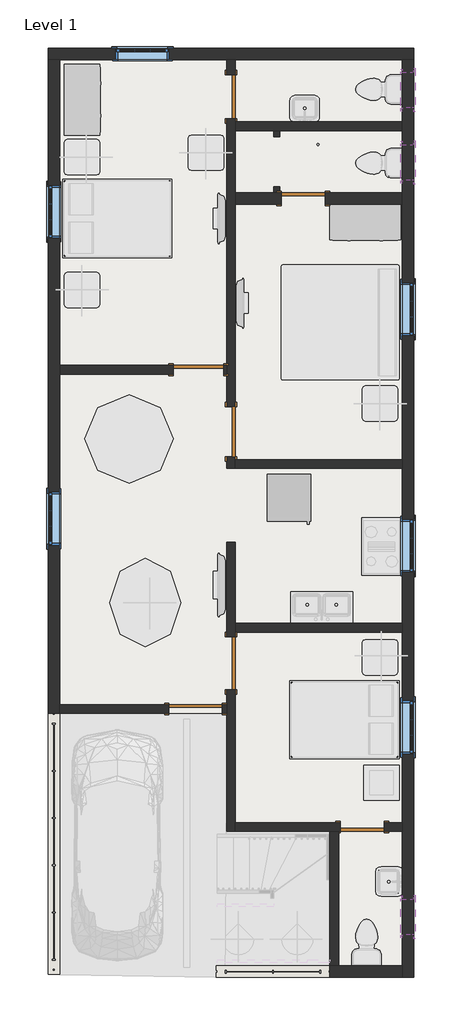
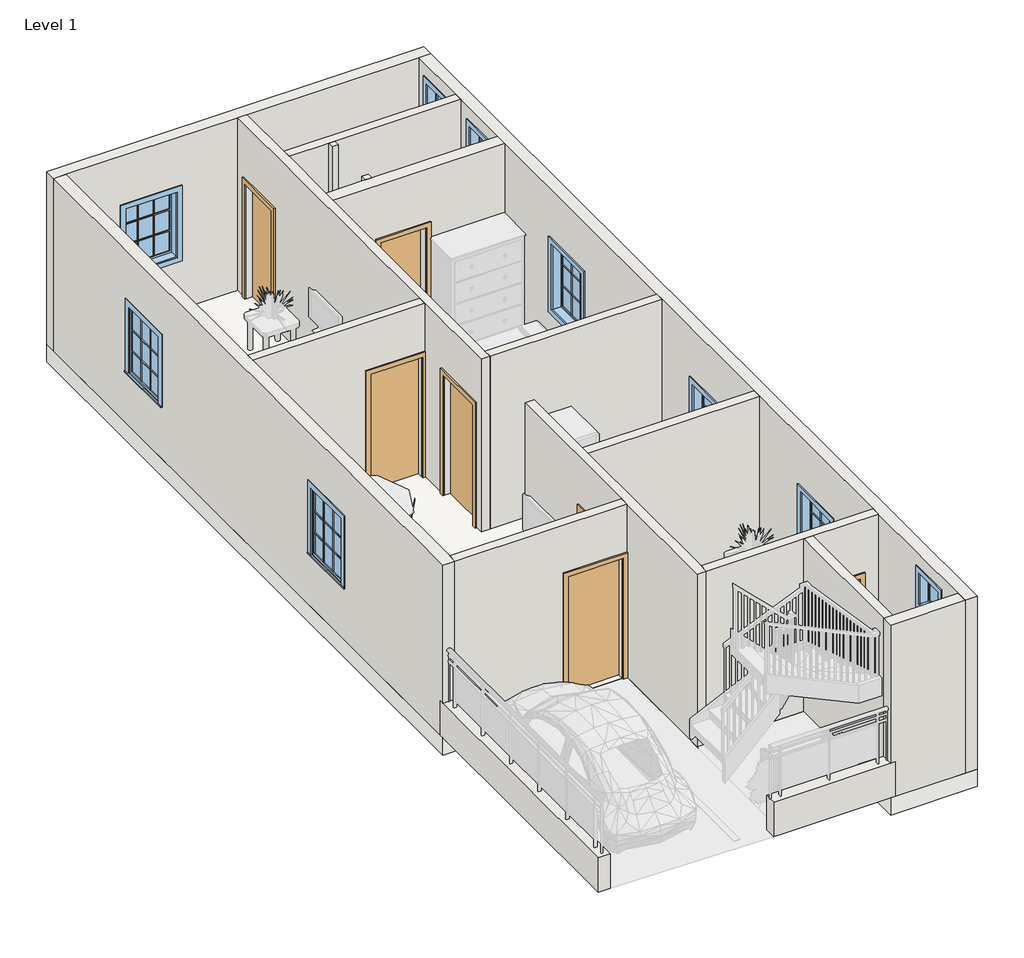
# One storey, part 1 of 3: 18 walls, 9 windows, 7 doors, 1 slab.
"""IFC4 building model written with IfcOpenShell, lengths in millimetres."""

from ifc_helpers import new_model, si_unit, frame, origin, origin_with_axes, place, context, project, spatial, polyline, outline, extrude, faceted_brep, transform, mapped, element, save
from components import door_059fdd7e, door_53b1b562, door_b6e9fca3, door_686f89d2, door_16372e1c, window_29c06734, window_e41d21a6

model = new_model("IFC4")

# Units and contexts
model_context = context("Model", 3, world=origin())
ifc_project = project(units=[si_unit("LENGTHUNIT", "METRE", prefix="MILLI")], contexts=[model_context])

# Site, building, storey
site = spatial("IfcSite", under=ifc_project)
building = spatial("IfcBuilding", under=site)
storey = spatial("IfcBuildingStorey", under=building, Name="Level 1", Elevation=0.0)

# Doors
placement = place(None, origin())
door_shape = door_059fdd7e(model_context)
element("IfcDoor", 1, ObjectType="Single-Flush : 30\" x 80\"", at=placement, inside=storey, context=model_context, shape_type="MappedRepresentation", body=[
    mapped(door_shape, transform((-11568.3112155, 12129.2104001, 0.0), x_axis=(0.0, -1.0, 0.0), y_axis=(1.0, 0.0, 0.0), z_axis=(0.0, 0.0, 1.0))),
])
element("IfcDoor", 2, ObjectType="Single-Flush : 30\" x 80\"", at=placement, inside=storey, context=model_context, shape_type="MappedRepresentation", body=[
    mapped(door_shape, transform((-9307.7112155, -443.7895999, 0.0), x_axis=(-1.0, 0.0, 0.0), y_axis=(0.0, -1.0, 0.0), z_axis=(0.0, 0.0, 1.0))),
])
door_2_shape = door_53b1b562(model_context)
element("IfcDoor", 3, ObjectType="Single-Flush : 30\" x 80\"", at=placement, inside=storey, context=model_context, shape_type="MappedRepresentation", body=[
    mapped(door_2_shape, transform((-10323.7112155, 10376.6104001, 0.0), x_axis=(-1.0, 0.0, 0.0), y_axis=(0.0, -1.0, 0.0), z_axis=(0.0, 0.0, 1.0))),
])
door_3_shape = door_b6e9fca3(model_context)
element("IfcDoor", 4, ObjectType="Single-Flush : 34\" x 84\"", at=placement, inside=storey, context=model_context, shape_type="MappedRepresentation", body=[
    mapped(door_3_shape, transform((-12127.1112155, 7430.2104001, 0.0), x_axis=(1.0, 0.0, 0.0), y_axis=(0.0, 1.0, 0.0), z_axis=(0.0, 0.0, 1.0))),
])
element("IfcDoor", 5, ObjectType="Single-Flush : 34\" x 84\"", at=placement, inside=storey, context=model_context, shape_type="MappedRepresentation", body=[
    mapped(door_3_shape, transform((-11568.3112155, 6363.4104001, 0.0), x_axis=(0.0, -1.0, 0.0), y_axis=(1.0, 0.0, 0.0), z_axis=(0.0, 0.0, 1.0))),
])
door_4_shape = door_686f89d2(model_context)
element("IfcDoor", 6, ObjectType="Single-Flush : 36\" x 84\"", at=placement, inside=storey, context=model_context, shape_type="MappedRepresentation", body=[
    mapped(door_4_shape, transform((-11568.3112155, 2375.6104001, 0.0), x_axis=(0.0, 1.0, 0.0), y_axis=(-1.0, 0.0, 0.0), z_axis=(0.0, 0.0, 1.0))),
])
door_5_shape = door_16372e1c(model_context)
element("IfcDoor", 7, ObjectType="Single-Flush : 36\" x 84\"", at=placement, inside=storey, context=model_context, shape_type="MappedRepresentation", body=[
    mapped(door_5_shape, transform((-12177.9112155, 1588.2104001, 0.0), x_axis=(1.0, 0.0, 0.0), y_axis=(0.0, 1.0, 0.0), z_axis=(0.0, 0.0, 1.0))),
])

# Slab
element("IfcSlab", 8, ObjectType="Generic - 12\"", at=placement, inside=storey, context=model_context, shape_type="SweptSolid", body=[
    extrude(outline(polyline([(-8418.7112155, 12967.4104001), (-8418.7112155, -3034.5895999), (-9866.5112155, -3034.5895999), (-9866.5112155, -519.9895999), (-11644.5112155, -519.9895999), (-11644.5112155, 1512.0104001), (-14717.9112155, 1512.0104001), (-14717.9112155, 12967.4104001), (-8418.7112155, 12967.4104001)])), frame((0.0, 0.0, -304.8), z_axis=(0.0, 0.0, 1.0), x_axis=(1.0, 0.0, 0.0)), (0.0, 0.0, 1.0), 304.8),
])

# Walls
element("IfcWall", 9, ObjectType="Generic - 2\"", at=placement, inside=storey, context=model_context, shape_type="Brep", body=[
    faceted_brep([(-14514.7112155, -2983.7895999, 0.0), (-14514.7112155, 1512.0104001, 0.0), (-14514.7112155, 1588.2104001, 0.0), (-14514.7112155, 1588.2104001, 609.6), (-14514.7112155, -2983.7895999, 609.6), (-14717.9112155, -2983.7895999, 0.0), (-14717.9112155, -2983.7895999, 609.6), (-14717.9112155, 1588.2104001, 609.6), (-14717.9112155, 1588.2104001, 0.0)], [[[0, 1, 2, 3, 4]], [[5, 6, 7, 8]], [[2, 1, 0, 5, 8]], [[3, 2, 8, 7]], [[4, 3, 7, 6]], [[0, 4, 6, 5]]]),
])
element("IfcWall", 10, ObjectType="Generic - 2\"", at=placement, inside=storey, context=model_context, shape_type="Brep", body=[
    faceted_brep([(-9790.3112155, -2831.3895999, 0.0), (-9866.5112155, -2831.3895999, 0.0), (-11822.3112155, -2831.3895999, 0.0), (-11822.3112155, -2831.3895999, 609.6), (-9790.3112155, -2831.3895999, 609.6), (-9790.3112155, -3034.5895999, 0.0), (-9790.3112155, -3034.5895999, 609.6), (-11822.3112155, -3034.5895999, 609.6), (-11822.3112155, -3034.5895999, 0.0)], [[[0, 1, 2, 3, 4]], [[5, 6, 7, 8]], [[2, 1, 0, 5, 8]], [[3, 2, 8, 7]], [[4, 3, 7, 6]], [[0, 4, 6, 5]]]),
])
element("IfcWall", 11, ObjectType="Generic - 8\"", at=placement, inside=storey, context=model_context, shape_type="Brep", body=[
    faceted_brep([(-14717.9112155, 12764.2104001, 0.0), (-14514.7112155, 12764.2104001, 0.0), (-11644.5112155, 12764.2104001, 0.0), (-11492.1112155, 12764.2104001, 0.0), (-8621.9112155, 12764.2104001, 0.0), (-8418.7112155, 12764.2104001, 0.0), (-8418.7112155, 12764.2104001, 3048.0), (-8621.9112155, 12764.2104001, 3048.0), (-11492.1112155, 12764.2104001, 3048.0), (-11644.5112155, 12764.2104001, 3048.0), (-14514.7112155, 12764.2104001, 3048.0), (-14717.9112155, 12764.2104001, 3048.0), (-12635.1112155, 12764.2104001, 2133.6), (-12635.1112155, 12764.2104001, 914.4), (-13549.5112155, 12764.2104001, 914.4), (-13549.5112155, 12764.2104001, 2133.6), (-14717.9112155, 12967.4104001, 0.0), (-14717.9112155, 12967.4104001, 3048.0), (-8418.7112155, 12967.4104001, 3048.0), (-8418.7112155, 12967.4104001, 0.0), (-12635.1112155, 12967.4104001, 2133.6), (-13549.5112155, 12967.4104001, 2133.6), (-13549.5112155, 12967.4104001, 914.4), (-12635.1112155, 12967.4104001, 914.4)], [[[0, 1, 2, 3, 4, 5, 6, 7, 8, 9, 10, 11], [12, 13, 14, 15]], [[16, 17, 18, 19], [20, 21, 22, 23]], [[5, 4, 3, 2, 1, 0, 16, 19]], [[6, 5, 19, 18]], [[0, 11, 17, 16]], [[13, 12, 20, 23]], [[14, 13, 23, 22]], [[15, 14, 22, 21]], [[12, 15, 21, 20]], [[11, 10, 9, 8, 7, 6, 18, 17]]]),
])
element("IfcWall", 12, ObjectType="Generic - 8\"", at=placement, inside=storey, context=model_context, shape_type="Brep", body=[
    faceted_brep([(-8621.9112155, 12764.2104001, 0.0), (-8621.9112155, 11697.4104001, 0.0), (-8621.9112155, 11545.0104001, 0.0), (-8621.9112155, 10478.2104001, 0.0), (-8621.9112155, 10275.0104001, 0.0), (-8621.9112155, 5880.8104001, 0.0), (-8621.9112155, 5728.4104001, 0.0), (-8621.9112155, 3061.4104001, 0.0), (-8621.9112155, 2909.0104001, 0.0), (-8621.9112155, -367.5895999, 0.0), (-8621.9112155, -519.9895999, 0.0), (-8621.9112155, -2831.3895999, 0.0), (-8621.9112155, -3034.5895999, 0.0), (-8621.9112155, -3034.5895999, 3048.0), (-8621.9112155, -2831.3895999, 3048.0), (-8621.9112155, -519.9895999, 3048.0), (-8621.9112155, -367.5895999, 3048.0), (-8621.9112155, 2909.0104001, 3048.0), (-8621.9112155, 3061.4104001, 3048.0), (-8621.9112155, 5728.4104001, 3048.0), (-8621.9112155, 5880.8104001, 3048.0), (-8621.9112155, 10275.0104001, 3048.0), (-8621.9112155, 10478.2104001, 3048.0), (-8621.9112155, 11545.0104001, 3048.0), (-8621.9112155, 11697.4104001, 3048.0), (-8621.9112155, 12764.2104001, 3048.0), (-8621.9112155, 813.5104001, 2133.6), (-8621.9112155, 813.5104001, 914.4), (-8621.9112155, 1727.9104001, 914.4), (-8621.9112155, 1727.9104001, 2133.6), (-8621.9112155, 3937.7104001, 2133.6), (-8621.9112155, 3937.7104001, 914.4), (-8621.9112155, 4852.1104001, 914.4), (-8621.9112155, 4852.1104001, 2133.6), (-8621.9112155, 8014.4104001, 2133.6), (-8621.9112155, 8014.4104001, 914.4), (-8621.9112155, 8928.8104001, 914.4), (-8621.9112155, 8928.8104001, 2133.6), (-8621.9112155, 11938.7104001, 2768.6), (-8621.9112155, 11938.7104001, 2159.0), (-8621.9112155, 12548.3104001, 2159.0), (-8621.9112155, 12548.3104001, 2768.6), (-8621.9112155, 10694.1104001, 2768.6), (-8621.9112155, 10694.1104001, 2159.0), (-8621.9112155, 11303.7104001, 2159.0), (-8621.9112155, 11303.7104001, 2768.6), (-8621.9112155, -2297.9895999, 2768.6), (-8621.9112155, -2297.9895999, 2159.0), (-8621.9112155, -1688.3895999, 2159.0), (-8621.9112155, -1688.3895999, 2768.6), (-8418.7112155, 12764.2104001, 0.0), (-8418.7112155, 12764.2104001, 3048.0), (-8418.7112155, -3034.5895999, 3048.0), (-8418.7112155, -3034.5895999, 0.0), (-8418.7112155, 813.5104001, 2133.6), (-8418.7112155, 1727.9104001, 2133.6), (-8418.7112155, 1727.9104001, 914.4), (-8418.7112155, 813.5104001, 914.4), (-8418.7112155, 3937.7104001, 2133.6), (-8418.7112155, 4852.1104001, 2133.6), (-8418.7112155, 4852.1104001, 914.4), (-8418.7112155, 3937.7104001, 914.4), (-8418.7112155, 8014.4104001, 2133.6), (-8418.7112155, 8928.8104001, 2133.6), (-8418.7112155, 8928.8104001, 914.4), (-8418.7112155, 8014.4104001, 914.4), (-8418.7112155, 11938.7104001, 2768.6), (-8418.7112155, 12548.3104001, 2768.6), (-8418.7112155, 12548.3104001, 2159.0), (-8418.7112155, 11938.7104001, 2159.0), (-8418.7112155, 10694.1104001, 2768.6), (-8418.7112155, 11303.7104001, 2768.6), (-8418.7112155, 11303.7104001, 2159.0), (-8418.7112155, 10694.1104001, 2159.0), (-8418.7112155, -2297.9895999, 2768.6), (-8418.7112155, -1688.3895999, 2768.6), (-8418.7112155, -1688.3895999, 2159.0), (-8418.7112155, -2297.9895999, 2159.0)], [[[0, 1, 2, 3, 4, 5, 6, 7, 8, 9, 10, 11, 12, 13, 14, 15, 16, 17, 18, 19, 20, 21, 22, 23, 24, 25], [26, 27, 28, 29], [30, 31, 32, 33], [34, 35, 36, 37], [38, 39, 40, 41], [42, 43, 44, 45], [46, 47, 48, 49]], [[50, 51, 52, 53], [54, 55, 56, 57], [58, 59, 60, 61], [62, 63, 64, 65], [66, 67, 68, 69], [70, 71, 72, 73], [74, 75, 76, 77]], [[12, 11, 10, 9, 8, 7, 6, 5, 4, 3, 2, 1, 0, 50, 53]], [[0, 25, 51, 50]], [[13, 12, 53, 52]], [[27, 26, 54, 57]], [[28, 27, 57, 56]], [[29, 28, 56, 55]], [[26, 29, 55, 54]], [[31, 30, 58, 61]], [[32, 31, 61, 60]], [[33, 32, 60, 59]], [[30, 33, 59, 58]], [[35, 34, 62, 65]], [[36, 35, 65, 64]], [[37, 36, 64, 63]], [[34, 37, 63, 62]], [[39, 38, 66, 69]], [[40, 39, 69, 68]], [[41, 40, 68, 67]], [[38, 41, 67, 66]], [[43, 42, 70, 73]], [[44, 43, 73, 72]], [[45, 44, 72, 71]], [[42, 45, 71, 70]], [[25, 24, 23, 22, 21, 20, 19, 18, 17, 16, 15, 14, 13, 52, 51]], [[47, 46, 74, 77]], [[48, 47, 77, 76]], [[49, 48, 76, 75]], [[46, 49, 75, 74]]]),
])
element("IfcWall", 13, ObjectType="Generic - 8\"", at=placement, inside=storey, context=model_context, shape_type="Brep", body=[
    faceted_brep([(-8621.9112155, -2831.3895999, 0.0), (-9714.1112155, -2831.3895999, 0.0), (-9790.3112155, -2831.3895999, 0.0), (-9790.3112155, -2831.3895999, 609.6), (-9866.5112155, -2831.3895999, 609.6), (-9866.5112155, -2831.3895999, 3048.0), (-9714.1112155, -2831.3895999, 3048.0), (-8621.9112155, -2831.3895999, 3048.0), (-8621.9112155, -3034.5895999, 0.0), (-8621.9112155, -3034.5895999, 3048.0), (-9866.5112155, -3034.5895999, 3048.0), (-9866.5112155, -3034.5895999, 609.6), (-9790.3112155, -3034.5895999, 609.6), (-9790.3112155, -3034.5895999, 0.0)], [[[0, 1, 2, 3, 4, 5, 6, 7]], [[8, 9, 10, 11, 12, 13]], [[2, 1, 0, 8, 13]], [[0, 7, 9, 8]], [[3, 2, 13, 12]], [[11, 4, 3, 12]], [[5, 4, 11, 10]], [[7, 6, 5, 10, 9]]]),
])
element("IfcWall", 14, ObjectType="Generic - 8\"", at=placement, inside=storey, context=model_context, shape_type="Brep", body=[
    faceted_brep([(-11492.1112155, 10275.0104001, 0.0), (-10704.7112155, 10275.0104001, 0.0), (-10704.7112155, 10275.0104001, 2032.0), (-9942.7112155, 10275.0104001, 2032.0), (-9942.7112155, 10275.0104001, 0.0), (-8621.9112155, 10275.0104001, 0.0), (-8621.9112155, 10275.0104001, 3048.0), (-11492.1112155, 10275.0104001, 3048.0), (-10704.7112155, 10478.2104001, 2032.0), (-10704.7112155, 10478.2104001, 0.0), (-10730.1112155, 10478.2104001, 0.0), (-10831.7112155, 10478.2104001, 0.0), (-11492.1112155, 10478.2104001, 0.0), (-11492.1112155, 10478.2104001, 3048.0), (-10831.7112155, 10478.2104001, 3048.0), (-10730.1112155, 10478.2104001, 3048.0), (-8621.9112155, 10478.2104001, 3048.0), (-8621.9112155, 10478.2104001, 0.0), (-9942.7112155, 10478.2104001, 0.0), (-9942.7112155, 10478.2104001, 2032.0)], [[[0, 1, 2, 3, 4, 5, 6, 7]], [[8, 9, 10, 11, 12, 13, 14, 15, 16, 17, 18, 19]], [[18, 17, 5, 4]], [[12, 11, 10, 9, 1, 0]], [[6, 5, 17, 16]], [[0, 7, 13, 12]], [[2, 1, 9, 8]], [[3, 2, 8, 19]], [[4, 3, 19, 18]], [[7, 6, 16, 15, 14, 13]]]),
])
element("IfcWall", 15, ObjectType="Generic - 8\"", at=placement, inside=storey, context=model_context, shape_type="Brep", body=[
    faceted_brep([(-14514.7112155, 1588.2104001, 0.0), (-14514.7112155, 1664.4104001, 0.0), (-14514.7112155, 7354.0104001, 0.0), (-14514.7112155, 7506.4104001, 0.0), (-14514.7112155, 12764.2104001, 0.0), (-14514.7112155, 12764.2104001, 3048.0), (-14514.7112155, 7506.4104001, 3048.0), (-14514.7112155, 7354.0104001, 3048.0), (-14514.7112155, 1664.4104001, 3048.0), (-14514.7112155, 1512.0104001, 3048.0), (-14514.7112155, 1512.0104001, 609.6), (-14514.7112155, 1588.2104001, 609.6), (-14514.7112155, 10605.2104001, 2133.6), (-14514.7112155, 10605.2104001, 914.4), (-14514.7112155, 9690.8104001, 914.4), (-14514.7112155, 9690.8104001, 2133.6), (-14514.7112155, 5322.0104001, 2133.6), (-14514.7112155, 5322.0104001, 914.4), (-14514.7112155, 4407.6104001, 914.4), (-14514.7112155, 4407.6104001, 2133.6), (-14717.9112155, 1588.2104001, 0.0), (-14717.9112155, 1588.2104001, 609.6), (-14717.9112155, 1512.0104001, 609.6), (-14717.9112155, 1512.0104001, 3048.0), (-14717.9112155, 12764.2104001, 3048.0), (-14717.9112155, 12764.2104001, 0.0), (-14717.9112155, 10605.2104001, 2133.6), (-14717.9112155, 9690.8104001, 2133.6), (-14717.9112155, 9690.8104001, 914.4), (-14717.9112155, 10605.2104001, 914.4), (-14717.9112155, 5322.0104001, 2133.6), (-14717.9112155, 4407.6104001, 2133.6), (-14717.9112155, 4407.6104001, 914.4), (-14717.9112155, 5322.0104001, 914.4)], [[[0, 1, 2, 3, 4, 5, 6, 7, 8, 9, 10, 11], [12, 13, 14, 15], [16, 17, 18, 19]], [[20, 21, 22, 23, 24, 25], [26, 27, 28, 29], [30, 31, 32, 33]], [[4, 3, 2, 1, 0, 20, 25]], [[5, 4, 25, 24]], [[12, 15, 27, 26]], [[15, 14, 28, 27]], [[14, 13, 29, 28]], [[13, 12, 26, 29]], [[16, 19, 31, 30]], [[19, 18, 32, 31]], [[18, 17, 33, 32]], [[17, 16, 30, 33]], [[0, 11, 21, 20]], [[10, 22, 21, 11]], [[10, 9, 23, 22]], [[9, 8, 7, 6, 5, 24, 23]]]),
])
element("IfcWall", 16, ObjectType="INNER 4\"", at=placement, inside=storey, context=model_context, shape_type="SweptSolid", body=[
    extrude(outline(polyline([(-10831.7112155, 11443.4104001), (-10831.7112155, 11545.0104001), (-10730.1112155, 11545.0104001), (-10730.1112155, 11443.4104001), (-10831.7112155, 11443.4104001)])), origin_with_axes(), (0.0, 0.0, 1.0), 3048.0),
])
element("IfcWall", 17, ObjectType="INNER 4\"", at=placement, inside=storey, context=model_context, shape_type="SweptSolid", body=[
    extrude(outline(polyline([(-10831.7112155, 10478.2104001), (-10831.7112155, 10579.8104001), (-10730.1112155, 10579.8104001), (-10730.1112155, 10478.2104001), (-10831.7112155, 10478.2104001)])), origin_with_axes(), (0.0, 0.0, 1.0), 3048.0),
])
element("IfcWall", 18, ObjectType="INNER 6\"", at=placement, inside=storey, context=model_context, shape_type="Brep", body=[
    faceted_brep([(-11644.5112155, 5931.6104001, 2133.6), (-11644.5112155, 5931.6104001, 0.0), (-11644.5112155, 5728.4104001, 0.0), (-11644.5112155, 5728.4104001, 3048.0), (-11644.5112155, 7354.0104001, 3048.0), (-11644.5112155, 7506.4104001, 3048.0), (-11644.5112155, 12764.2104001, 3048.0), (-11644.5112155, 12764.2104001, 0.0), (-11644.5112155, 12510.2104001, 0.0), (-11644.5112155, 12510.2104001, 2032.0), (-11644.5112155, 11748.2104001, 2032.0), (-11644.5112155, 11748.2104001, 0.0), (-11644.5112155, 7506.4104001, 0.0), (-11644.5112155, 7354.0104001, 0.0), (-11644.5112155, 6795.2104001, 0.0), (-11644.5112155, 6795.2104001, 2133.6), (-11492.1112155, 5728.4104001, 0.0), (-11492.1112155, 5880.8104001, 0.0), (-11492.1112155, 5931.6104001, 0.0), (-11492.1112155, 5931.6104001, 2133.6), (-11492.1112155, 6795.2104001, 2133.6), (-11492.1112155, 6795.2104001, 0.0), (-11492.1112155, 10275.0104001, 0.0), (-11492.1112155, 10478.2104001, 0.0), (-11492.1112155, 11545.0104001, 0.0), (-11492.1112155, 11697.4104001, 0.0), (-11492.1112155, 11748.2104001, 0.0), (-11492.1112155, 11748.2104001, 2032.0), (-11492.1112155, 12510.2104001, 2032.0), (-11492.1112155, 12510.2104001, 0.0), (-11492.1112155, 12764.2104001, 0.0), (-11492.1112155, 12764.2104001, 3048.0), (-11492.1112155, 11697.4104001, 3048.0), (-11492.1112155, 11545.0104001, 3048.0), (-11492.1112155, 10478.2104001, 3048.0), (-11492.1112155, 10275.0104001, 3048.0), (-11492.1112155, 5880.8104001, 3048.0), (-11492.1112155, 5728.4104001, 3048.0)], [[[0, 1, 2, 3, 4, 5, 6, 7, 8, 9, 10, 11, 12, 13, 14, 15]], [[16, 17, 18, 19, 20, 21, 22, 23, 24, 25, 26, 27, 28, 29, 30, 31, 32, 33, 34, 35, 36, 37]], [[8, 7, 30, 29]], [[2, 1, 18, 17, 16]], [[14, 13, 12, 11, 26, 25, 24, 23, 22, 21]], [[7, 6, 31, 30]], [[27, 26, 11, 10]], [[28, 27, 10, 9]], [[29, 28, 9, 8]], [[19, 18, 1, 0]], [[20, 19, 0, 15]], [[21, 20, 15, 14]], [[3, 2, 16, 37]], [[6, 5, 4, 3, 37, 36, 35, 34, 33, 32, 31]]]),
])
element("IfcWall", 19, ObjectType="INNER 6\"", at=placement, inside=storey, context=model_context, shape_type="Brep", body=[
    faceted_brep([(-11492.1112155, 11545.0104001, 0.0), (-10831.7112155, 11545.0104001, 0.0), (-10730.1112155, 11545.0104001, 0.0), (-8621.9112155, 11545.0104001, 0.0), (-8621.9112155, 11545.0104001, 3048.0), (-10730.1112155, 11545.0104001, 3048.0), (-10831.7112155, 11545.0104001, 3048.0), (-11492.1112155, 11545.0104001, 3048.0), (-11492.1112155, 11697.4104001, 0.0), (-11492.1112155, 11697.4104001, 3048.0), (-8621.9112155, 11697.4104001, 3048.0), (-8621.9112155, 11697.4104001, 0.0)], [[[0, 1, 2, 3, 4, 5, 6, 7]], [[8, 9, 10, 11]], [[3, 2, 1, 0, 8, 11]], [[4, 3, 11, 10]], [[0, 7, 9, 8]], [[7, 6, 5, 4, 10, 9]]]),
])
element("IfcWall", 20, ObjectType="INNER 6\"", at=placement, inside=storey, context=model_context, shape_type="SweptSolid", body=[
    extrude(outline(polyline([(-8621.9112155, 5728.4104001), (-11492.1112155, 5728.4104001), (-11492.1112155, 5880.8104001), (-8621.9112155, 5880.8104001), (-8621.9112155, 5728.4104001)])), origin_with_axes(), (0.0, 0.0, 1.0), 3048.0),
])
element("IfcWall", 21, ObjectType="INNER 6\"", at=placement, inside=storey, context=model_context, shape_type="SweptSolid", body=[
    extrude(outline(polyline([(2133.6, -11695.3112155), (0.0, -11695.3112155), (0.0, -11644.5112155), (3048.0, -11644.5112155), (3048.0, -14514.7112155), (0.0, -14514.7112155), (0.0, -12558.9112155), (2133.6, -12558.9112155), (2133.6, -11695.3112155)])), frame((0.0, 7354.0104001, 0.0), z_axis=(0.0, 1.0, 0.0), x_axis=(0.0, 0.0, 1.0)), (0.0, 0.0, 1.0), 152.4),
])
element("IfcWall", 22, ObjectType="INNER 6\"", at=placement, inside=storey, context=model_context, shape_type="Brep", body=[
    faceted_brep([(-11720.7112155, 1512.0104001, 2133.6), (-11720.7112155, 1512.0104001, 0.0), (-11644.5112155, 1512.0104001, 0.0), (-11644.5112155, 1512.0104001, 3048.0), (-14514.7112155, 1512.0104001, 3048.0), (-14514.7112155, 1512.0104001, 609.6), (-14514.7112155, 1512.0104001, 0.0), (-12635.1112155, 1512.0104001, 0.0), (-12635.1112155, 1512.0104001, 2133.6), (-11644.5112155, 1664.4104001, 0.0), (-11720.7112155, 1664.4104001, 0.0), (-11720.7112155, 1664.4104001, 2133.6), (-12635.1112155, 1664.4104001, 2133.6), (-12635.1112155, 1664.4104001, 0.0), (-14514.7112155, 1664.4104001, 0.0), (-14514.7112155, 1664.4104001, 3048.0), (-11644.5112155, 1664.4104001, 3048.0), (-14514.7112155, 1588.2104001, 0.0)], [[[0, 1, 2, 3, 4, 5, 6, 7, 8]], [[9, 10, 11, 12, 13, 14, 15, 16]], [[7, 6, 17, 14, 13]], [[2, 1, 10, 9]], [[3, 2, 9, 16]], [[11, 10, 1, 0]], [[12, 11, 0, 8]], [[13, 12, 8, 7]], [[4, 15, 14, 17, 6, 5]], [[4, 3, 16, 15]]]),
])
element("IfcWall", 23, ObjectType="INNER 6\"", at=placement, inside=storey, context=model_context, shape_type="SweptSolid", body=[
    extrude(outline(polyline([(-8621.9112155, 2909.0104001), (-11492.1112155, 2909.0104001), (-11492.1112155, 3061.4104001), (-8621.9112155, 3061.4104001), (-8621.9112155, 2909.0104001)])), origin_with_axes(), (0.0, 0.0, 1.0), 3048.0),
])
element("IfcWall", 24, ObjectType="INNER 6\"", at=placement, inside=storey, context=model_context, shape_type="Brep", body=[
    faceted_brep([(-11492.1112155, -519.9895999, 0.0), (-9866.5112155, -519.9895999, 0.0), (-9714.1112155, -519.9895999, 0.0), (-9688.7112155, -519.9895999, 0.0), (-9688.7112155, -519.9895999, 2032.0), (-8926.7112155, -519.9895999, 2032.0), (-8926.7112155, -519.9895999, 0.0), (-8621.9112155, -519.9895999, 0.0), (-8621.9112155, -519.9895999, 3048.0), (-9714.1112155, -519.9895999, 3048.0), (-9866.5112155, -519.9895999, 3048.0), (-11492.1112155, -519.9895999, 3048.0), (-9688.7112155, -367.5895999, 2032.0), (-9688.7112155, -367.5895999, 0.0), (-11492.1112155, -367.5895999, 0.0), (-11492.1112155, -367.5895999, 3048.0), (-8621.9112155, -367.5895999, 3048.0), (-8621.9112155, -367.5895999, 0.0), (-8926.7112155, -367.5895999, 0.0), (-8926.7112155, -367.5895999, 2032.0)], [[[0, 1, 2, 3, 4, 5, 6, 7, 8, 9, 10, 11]], [[12, 13, 14, 15, 16, 17, 18, 19]], [[18, 17, 7, 6]], [[14, 13, 3, 2, 1, 0]], [[0, 11, 15, 14]], [[8, 7, 17, 16]], [[4, 3, 13, 12]], [[5, 4, 12, 19]], [[6, 5, 19, 18]], [[11, 10, 9, 8, 16, 15]]]),
])
element("IfcWall", 25, ObjectType="INNER 6\"", at=placement, inside=storey, context=model_context, shape_type="Brep", body=[
    faceted_brep([(-9866.5112155, -519.9895999, 0.0), (-9866.5112155, -2831.3895999, 0.0), (-9866.5112155, -2831.3895999, 609.6), (-9866.5112155, -2831.3895999, 3048.0), (-9866.5112155, -519.9895999, 3048.0), (-9714.1112155, -519.9895999, 0.0), (-9714.1112155, -519.9895999, 3048.0), (-9714.1112155, -2831.3895999, 3048.0), (-9714.1112155, -2831.3895999, 0.0), (-9790.3112155, -2831.3895999, 0.0)], [[[0, 1, 2, 3, 4]], [[5, 6, 7, 8]], [[1, 0, 5, 8, 9]], [[0, 4, 6, 5]], [[1, 9, 8, 7, 3, 2]], [[4, 3, 7, 6]]]),
])
element("IfcWall", 26, ObjectType="INNER 6\"", at=placement, inside=storey, context=model_context, shape_type="Brep", body=[
    faceted_brep([(-11644.5112155, 4458.4104001, 0.0), (-11644.5112155, 2832.8104001, 0.0), (-11644.5112155, 2832.8104001, 2133.6), (-11644.5112155, 1918.4104001, 2133.6), (-11644.5112155, 1918.4104001, 0.0), (-11644.5112155, 1664.4104001, 0.0), (-11644.5112155, 1512.0104001, 0.0), (-11644.5112155, -519.9895999, 0.0), (-11644.5112155, -519.9895999, 3048.0), (-11644.5112155, 1512.0104001, 3048.0), (-11644.5112155, 1664.4104001, 3048.0), (-11644.5112155, 4458.4104001, 3048.0), (-11492.1112155, 2832.8104001, 2133.6), (-11492.1112155, 2832.8104001, 0.0), (-11492.1112155, 2909.0104001, 0.0), (-11492.1112155, 3061.4104001, 0.0), (-11492.1112155, 4458.4104001, 0.0), (-11492.1112155, 4458.4104001, 3048.0), (-11492.1112155, 3061.4104001, 3048.0), (-11492.1112155, 2909.0104001, 3048.0), (-11492.1112155, -367.5895999, 3048.0), (-11492.1112155, -519.9895999, 3048.0), (-11492.1112155, -519.9895999, 0.0), (-11492.1112155, -367.5895999, 0.0), (-11492.1112155, 1918.4104001, 0.0), (-11492.1112155, 1918.4104001, 2133.6)], [[[0, 1, 2, 3, 4, 5, 6, 7, 8, 9, 10, 11]], [[12, 13, 14, 15, 16, 17, 18, 19, 20, 21, 22, 23, 24, 25]], [[24, 23, 22, 7, 6, 5, 4]], [[16, 15, 14, 13, 1, 0]], [[0, 11, 17, 16]], [[8, 7, 22, 21]], [[2, 1, 13, 12]], [[3, 2, 12, 25]], [[4, 3, 25, 24]], [[11, 10, 9, 8, 21, 20, 19, 18, 17]]]),
])

# Windows
window_shape = window_29c06734(model_context)
element("IfcWindow", 27, ObjectType="Casement 3x3 with Trim : 36\" x 48\"", at=placement, inside=storey, context=model_context, shape_type="MappedRepresentation", body=[
    mapped(window_shape, transform((-13092.3112155, 12865.8104001, 0.0), x_axis=(1.0, 0.0, 0.0), y_axis=(0.0, 1.0, 0.0), z_axis=(0.0, 0.0, 1.0))),
])
element("IfcWindow", 28, ObjectType="Casement 3x3 with Trim : 36\" x 48\"", at=placement, inside=storey, context=model_context, shape_type="MappedRepresentation", body=[
    mapped(window_shape, transform((-14616.3112155, 10148.0104001, 0.0), x_axis=(0.0, 1.0, 0.0), y_axis=(-1.0, 0.0, 0.0), z_axis=(0.0, 0.0, 1.0))),
])
element("IfcWindow", 29, ObjectType="Casement 3x3 with Trim : 36\" x 48\"", at=placement, inside=storey, context=model_context, shape_type="MappedRepresentation", body=[
    mapped(window_shape, transform((-14616.3112155, 4864.8104001, 0.0), x_axis=(0.0, 1.0, 0.0), y_axis=(-1.0, 0.0, 0.0), z_axis=(0.0, 0.0, 1.0))),
])
element("IfcWindow", 30, ObjectType="Casement 3x3 with Trim : 36\" x 48\"", at=placement, inside=storey, context=model_context, shape_type="MappedRepresentation", body=[
    mapped(window_shape, transform((-8520.3112155, 1270.7104001, 0.0), x_axis=(0.0, -1.0, 0.0), y_axis=(1.0, 0.0, 0.0), z_axis=(0.0, 0.0, 1.0))),
])
element("IfcWindow", 31, ObjectType="Casement 3x3 with Trim : 36\" x 48\"", at=placement, inside=storey, context=model_context, shape_type="MappedRepresentation", body=[
    mapped(window_shape, transform((-8520.3112155, 4394.9104001, 0.0), x_axis=(0.0, -1.0, 0.0), y_axis=(1.0, 0.0, 0.0), z_axis=(0.0, 0.0, 1.0))),
])
element("IfcWindow", 32, ObjectType="Casement 3x3 with Trim : 36\" x 48\"", at=placement, inside=storey, context=model_context, shape_type="MappedRepresentation", body=[
    mapped(window_shape, transform((-8520.3112155, 8471.6104001, 0.0), x_axis=(0.0, -1.0, 0.0), y_axis=(1.0, 0.0, 0.0), z_axis=(0.0, 0.0, 1.0))),
])
window_2_shape = window_e41d21a6(model_context)
element("IfcWindow", 33, ObjectType="Transom with Trim : 24\" x 24\"", at=placement, inside=storey, context=model_context, shape_type="MappedRepresentation", body=[
    mapped(window_2_shape, transform((-8520.3112155, 12205.4104001, 0.0), x_axis=(0.0, -1.0, 0.0), y_axis=(1.0, 0.0, 0.0), z_axis=(0.0, 0.0, 1.0))),
])
element("IfcWindow", 34, ObjectType="Transom with Trim : 24\" x 24\"", at=placement, inside=storey, context=model_context, shape_type="MappedRepresentation", body=[
    mapped(window_2_shape, transform((-8520.3112155, 10960.8104001, 0.0), x_axis=(0.0, -1.0, 0.0), y_axis=(1.0, 0.0, 0.0), z_axis=(0.0, 0.0, 1.0))),
])
element("IfcWindow", 35, ObjectType="Transom with Trim : 24\" x 24\"", at=placement, inside=storey, context=model_context, shape_type="MappedRepresentation", body=[
    mapped(window_2_shape, transform((-8520.3112155, -2031.2895999, 0.0), x_axis=(0.0, -1.0, 0.0), y_axis=(1.0, 0.0, 0.0), z_axis=(0.0, 0.0, 1.0))),
])

save(model, "model.ifc")

# Revit data of these elements
# Type "Single-Flush : 30\" x 80\""
#   Type Mark = "5"
#   Construction Type Id = "MDOOR"
#   Assembly Code = "C1020"
#   Analytic Construction = "Metal"
#   Thickness = 0' - 2"
#   Heat Transfer Coefficient (U) = 0.651978 BTU/(h·ft²·°F)
#   Height = 6' - 8"
#   Trim Projection Ext = 0' - 1"
#   Trim Projection Int = 0' - 1"
#   Trim Width = 0' - 3"
#   Width = 2' - 6"
#   Define Thermal Properties by = 1
#   Door Material = Door - Panel
#   Frame Material = Door - Frame
#   Visual Light Transmittance = 0
#   Solar Heat Gain Coefficient = 0
#   Function = (empty or 0)
#   Wall Closure = (empty or 0)
# Type "Single-Flush : 34\" x 84\""
#   Type Mark = "2"
#   Construction Type Id = "MDOOR"
#   Assembly Code = "C1020"
#   Analytic Construction = "Metal"
#   Thickness = 0' - 2"
#   Heat Transfer Coefficient (U) = 0.651978 BTU/(h·ft²·°F)
#   Height = 7' - 0"
#   Trim Projection Ext = 0' - 1"
#   Trim Projection Int = 0' - 1"
#   Trim Width = 0' - 3"
#   Width = 2' - 10"
#   Define Thermal Properties by = 1
#   Door Material = Door - Panel
#   Frame Material = Door - Frame
#   Visual Light Transmittance = 0
#   Solar Heat Gain Coefficient = 0
#   Function = (empty or 0)
#   Wall Closure = (empty or 0)
# Type "Single-Flush : 36\" x 84\""
#   Type Mark = "1"
#   Construction Type Id = "MDOOR"
#   Assembly Code = "C1020"
#   Analytic Construction = "Metal"
#   Thickness = 0' - 2"
#   Heat Transfer Coefficient (U) = 0.651978 BTU/(h·ft²·°F)
#   Height = 7' - 0"
#   Trim Projection Ext = 0' - 1"
#   Trim Projection Int = 0' - 1"
#   Trim Width = 0' - 3"
#   Width = 3' - 0"
#   Define Thermal Properties by = 1
#   Door Material = Door - Panel
#   Frame Material = Door - Frame
#   Visual Light Transmittance = 0
#   Solar Heat Gain Coefficient = 0
#   Function = (empty or 0)
#   Wall Closure = (empty or 0)
# Type "Generic - 12\""
#   Assembly Code = "B1010"
#   Function = 0
#   Layers, outside or top first: 1' - 0" no material (function 1)
# Type "Generic - 2\""
#   Assembly Code = "B2010"
#   Layers, outside or top first: 0' - 8" "Birch" (function 1)
# Type "Generic - 8\""
#   Assembly Code = "B2010"
#   Layers, outside or top first: 0' - 8" "Brick, Common" (function 1)
# Type "INNER 4\""
#   Assembly Code = "B2010"
#   Layers, outside or top first: 0' - 4" no material (function 1)
# Type "INNER 6\""
#   Assembly Code = "B2010"
#   Layers, outside or top first: 0' - 6" "Brick, Common" (function 1)
# Type "Casement 3x3 with Trim : 36\" x 48\""
#   Type Mark = "10"
#   Construction Type Id = "GSP4R"
#   Assembly Code = "B2020100"
#   Analytic Construction = "1/8 in Pilkington single glazing"
#   Visual Light Transmittance = 0.9
#   Solar Heat Gain Coefficient = 0.78
#   Heat Transfer Coefficient (U) = 0.6496 BTU/(h·ft²·°F)
#   Height = 4' - 0"
#   Default Sill Height = 3' - 0"
#   Trim Projection - Ext. = 0' - 0 1/2"
#   Trim Projection - Int. = 0' - 0 3/4"
#   Trim Width - Exterior = 0' - 3 1/2"
#   Trim Width - Interior = 0' - 3 1/2"
#   Width = 3' - 0"
#   Window Inset = 0' - 0 3/4"
#   Define Thermal Properties by = 1
#   Glass Pane Material = Glass
#   Sash Material = Sash
#   Trim Exterior Material = Trim
#   Trim Interior Material = Trim
#   Wall Closure = (empty or 0)
# Type "Transom with Trim : 24\" x 24\""
#   Type Mark = "13"
#   Construction Type Id = "GSP4R"
#   Assembly Code = "B2020100"
#   Analytic Construction = "1/8 in Pilkington single glazing"
#   Visual Light Transmittance = 0.9
#   Solar Heat Gain Coefficient = 0.78
#   Heat Transfer Coefficient (U) = 0.6496 BTU/(h·ft²·°F)
#   Height = 2' - 0"
#   Default Sill Height = 7' - 1"
#   Trim Projection - Ext. = 0' - 0 1/2"
#   Trim Projection - Int. = 0' - 0 3/4"
#   Trim Width - Exterior = 0' - 3 1/2"
#   Trim Width - Interior = 0' - 3 1/2"
#   Width = 2' - 0"
#   Window Inset = 0' - 0 3/4"
#   Define Thermal Properties by = 1
#   Glass Pane Material = Glass
#   Sash Material = Sash
#   Trim Exterior Material = Trim
#   Trim Interior Material = Trim
#   Wall Closure = (empty or 0)
# Elements 1, 2, 3 (IfcDoor, "Single-Flush : 30\" x 80\"")
#   Phase Created = New Construction
#   Materials on its faces: "Door - Frame", "Door - Panel"
# Elements 4, 5 (IfcDoor, "Single-Flush : 34\" x 84\"")
#   Phase Created = New Construction
#   Materials on its faces: "Door - Frame", "Door - Panel"
# Elements 6, 7 (IfcDoor, "Single-Flush : 36\" x 84\"")
#   Phase Created = New Construction
#   Materials on its faces: "Door - Frame", "Door - Panel"
# Element 8 (IfcSlab, "Generic - 12\"")
#   Height Offset From Level = 0' - 0"
#   Phase Created = New Construction
#   Materials on its faces: "Default Floor"
# Elements 9, 10 (IfcWall, "Generic - 2\"")
#   Top Offset = 0' - 0"
#   Base Offset = 0' - 0"
#   Unconnected Height = 2' - 0"
#   wall height = 2' - 0"
#   Phase Created = New Construction
#   Base Constraint = Level 1
#   Materials on its faces: "Birch"
# Elements 11, 12, 13, 14, 15 (IfcWall, "Generic - 8\"")
#   Top Offset = 0' - 0"
#   Base Offset = 0' - 0"
#   Unconnected Height = 10' - 0"
#   wall height = 10' - 0"
#   Phase Created = New Construction
#   Base Constraint = Level 1
#   Materials on its faces: "Brick, Common"
# Elements 16, 17 (IfcWall, "INNER 4\"")
#   Top Offset = 0' - 0"
#   Base Offset = 0' - 0"
#   Unconnected Height = 10' - 0"
#   wall height = 10' - 0"
#   Phase Created = New Construction
#   Base Constraint = Level 1
#   Materials on its faces: "Default Wall"
# Elements 18, 19, 20, 21, 22, 23, 24, 25, 26 (IfcWall, "INNER 6\"")
#   Top Offset = 0' - 0"
#   Base Offset = 0' - 0"
#   Unconnected Height = 10' - 0"
#   wall height = 10' - 0"
#   Phase Created = New Construction
#   Base Constraint = Level 1
#   Materials on its faces: "Brick, Common"
# Element 27 (IfcWindow, "Casement 3x3 with Trim : 36\" x 48\"")
#   Mark = "1"
#   Phase Created = New Construction
#   Materials on its faces: "Sash", "Glass", "Trim"
# Element 28 (IfcWindow, "Casement 3x3 with Trim : 36\" x 48\"")
#   Mark = "2"
#   Phase Created = New Construction
#   Materials on its faces: "Sash", "Glass", "Trim"
# Element 29 (IfcWindow, "Casement 3x3 with Trim : 36\" x 48\"")
#   Mark = "3"
#   Phase Created = New Construction
#   Materials on its faces: "Sash", "Glass", "Trim"
# Element 30 (IfcWindow, "Casement 3x3 with Trim : 36\" x 48\"")
#   Mark = "4"
#   Phase Created = New Construction
#   Materials on its faces: "Sash", "Glass", "Trim"
# Element 31 (IfcWindow, "Casement 3x3 with Trim : 36\" x 48\"")
#   Mark = "5"
#   Phase Created = New Construction
#   Materials on its faces: "Sash", "Glass", "Trim"
# Element 32 (IfcWindow, "Casement 3x3 with Trim : 36\" x 48\"")
#   Mark = "6"
#   Phase Created = New Construction
#   Materials on its faces: "Sash", "Glass", "Trim"
# Element 33 (IfcWindow, "Transom with Trim : 24\" x 24\"")
#   Mark = "7"
#   Phase Created = New Construction
#   Materials on its faces: "Sash", "Trim", "Glass"
# Element 34 (IfcWindow, "Transom with Trim : 24\" x 24\"")
#   Mark = "8"
#   Phase Created = New Construction
#   Materials on its faces: "Sash", "Trim", "Glass"
# Element 35 (IfcWindow, "Transom with Trim : 24\" x 24\"")
#   Mark = "10"
#   Phase Created = New Construction
#   Materials on its faces: "Sash", "Trim", "Glass"
# Materials
#   "Door - Panel": class "Wood", colour RGB 210 159 95, transparency 0
#   "Door - Frame": colour RGB 118 70 51, transparency 0
#   "Birch": class "Wood", colour RGB 224 178 126, transparency 0, Description = "Betula Alleghaniensis", Cost = 0
#   "Brick, Common": class "Masonry", colour RGB 170 98 104, transparency 0, Description = "Common brick", Cost = 0
#   "Glass": class "Glass", colour RGB 0 128 192, transparency 0.75, Description = "Soda Lime Glass", Cost = 0
#   "Sash": class "Wood", colour RGB 224 178 126, transparency 0
#   "Trim": class "Wood", colour RGB 224 178 126, transparency 0
#   "Default Floor": colour RGB 128 128 128, transparency 0
#   "Default Wall": colour RGB 128 128 128, transparency 0
# Room at (-9973.013, 4277.809) mm, phase "New Construction", upper level "Level 1", upper offset 10' - 0", lower offset 0' - 0"
#   Number = "8"
#   Name = "KITCHEN"
# Room at (-13382.446, 4561.883) mm, phase "New Construction", upper level "Level 1", upper offset 10' - 0", lower offset 0' - 0"
#   Number = "6"
#   Name = "HALL"
# Room at (-10231.722, 4561.883) mm, phase "New Construction", upper level "Level 1", upper offset 10' - 0", lower offset 0' - 0"
#   Number = "7"
#   Name = "Room"
# Room at (-13205.934, 9986.799) mm, phase "New Construction", upper level "Level 1", upper offset 10' - 0", lower offset 0' - 0"
#   Number = "1"
#   Name = "BEDROOM"
# Room at (-10231.722, 12121.663) mm, phase "New Construction", upper level "Level 1", upper offset 10' - 0", lower offset 0' - 0"
#   Number = "2"
#   Name = "TOILET"
# Room at (-9976.269, 10748.359) mm, phase "New Construction", upper level "Level 1", upper offset 10' - 0", lower offset 0' - 0"
#   Number = "3"
#   Name = "TOILET"
# Room at (-11026.583, 10859.507) mm, phase "New Construction", upper level "Level 1", upper offset 10' - 0", lower offset 0' - 0"
#   Number = "4"
# Room at (-10010.701, 1135.065) mm, phase "New Construction", upper level "Level 1", upper offset 10' - 0", lower offset 0' - 0"
#   Number = "9"
#   Name = "BEDROOM"
# Room at (-9160.166, -1403.606) mm, phase "New Construction", upper level "Level 1", upper offset 10' - 0", lower offset 0' - 0"
#   Number = "10"
#   Name = "TOILET"
# Room at (-13442.588, -884.888) mm, phase "New Construction", upper level "Level 1", upper offset 10' - 0", lower offset 0' - 0"
#   Number = "11"
#   Name = "PARKING"
# Room at (-9933.717, 7890.853) mm, phase "New Construction", upper level "Level 1", upper offset 10' - 0", lower offset 0' - 0"
#   Number = "5"
#   Name = "BEDROOM"
